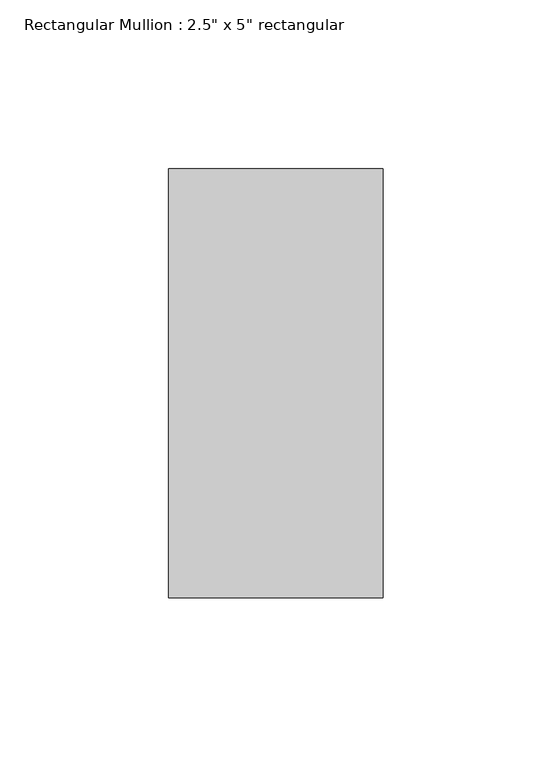
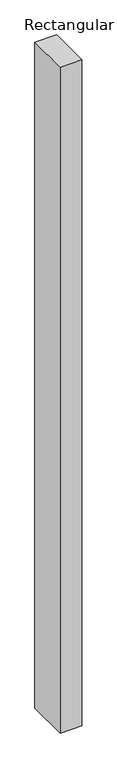
"""IFC4 building model written with IfcOpenShell, lengths in millimetres: member geometry."""

from ifc_helpers import new_model, si_unit, frame, origin, place, context, project, spatial, polyline, outline, extrude, source, transform, mapped, element, save


def member_b399a46d(model_context):
    return source(origin(), model_context, "Body", "SweptSolid", [
        extrude(outline(polyline([(0.0, 63.5), (0.0, -63.5), (-63.5, -63.5), (-63.5, 63.5), (0.0, 63.5)])), frame((0.0, 0.0, -2054.3954044), z_axis=(0.0, 0.0, 1.0), x_axis=(1.0, 0.0, 0.0)), (0.0, 0.0, 1.0), 2054.3954044),
    ])


if __name__ == "__main__":
    model = new_model("IFC4")
    model_context = context("Model", 3, world=origin())
    ifc_project = project(units=[si_unit("LENGTHUNIT", "METRE", prefix="MILLI")], contexts=[model_context])
    site = spatial("IfcSite", under=ifc_project)
    building = spatial("IfcBuilding", under=site)
    placement = place(None, origin())
    member_shape = member_b399a46d(model_context)
    element("IfcMember", 1, ObjectType="Rectangular Mullion : 2.5\" x 5\" rectangular", at=placement, inside=building, context=model_context, shape_type="MappedRepresentation", body=[
        mapped(member_shape, transform((0.0, 0.0, 0.0), x_axis=(1.0, 0.0, 0.0), y_axis=(0.0, 1.0, 0.0), z_axis=(0.0, 0.0, 1.0))),
    ])
    save(model, "model.ifc")

# Revit data of these elements
# Type "Rectangular Mullion : 2.5\" x 5\" rectangular"
#   built-in parameter 1007304 = 0.416667 (stored number, unit not read)
#   built-in parameter 1007301 = 0.104167 (stored number, unit not read)
#   built-in parameter 1007300 = 0.104167 (stored number, unit not read)
# Element 1 (IfcMember, "Rectangular Mullion : 2.5\" x 5\" rectangular")
#   Materials on its faces: "Aluminum"
# Materials
#   "Aluminum": class "Metal", colour RGB 247 247 247, transparency 0, Description = "Aluminum 6061", Cost = 0
